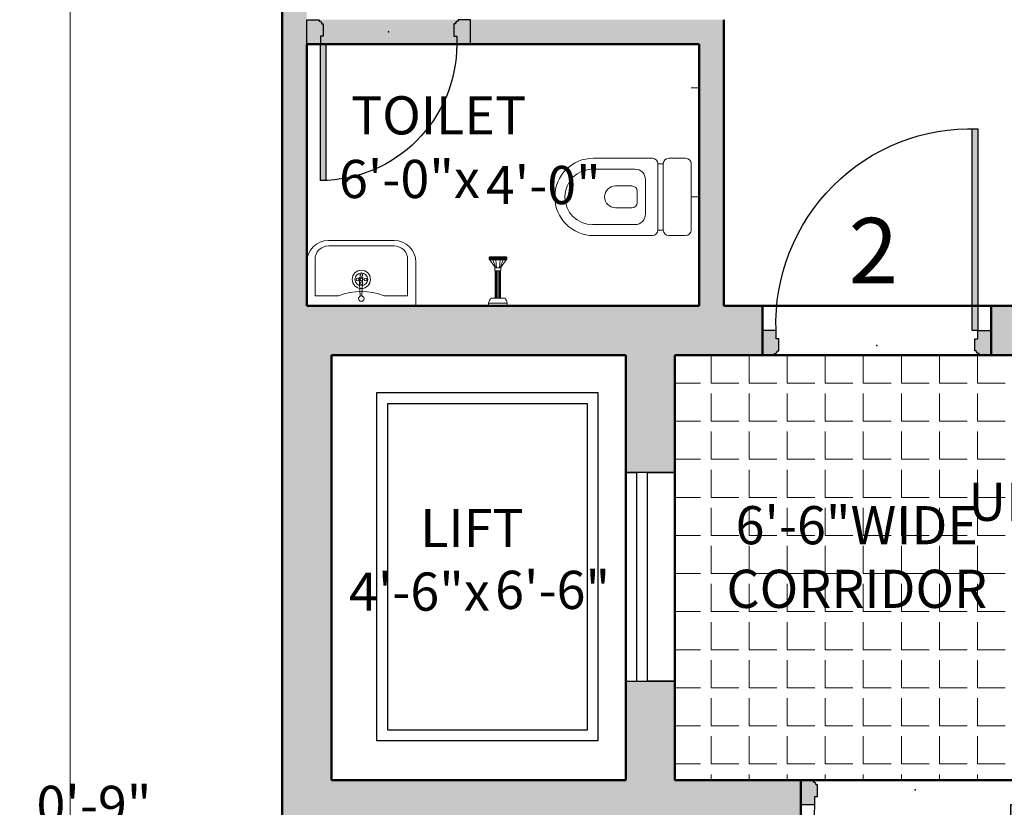
# Model space of a CAD drawing. Units: inches. Extents: x 4508 to 5907, y 877 to 1592.
# Tile 15 of 20: x 5203 to 5383, y 1298 to 1443. Entities that reach past the tile are written whole.
import ezdxf

# ---------------------------------------------------------------- set-up
doc = ezdxf.new("R2010")
doc.units = ezdxf.units.IN
doc.layers.get('DEFPOINTS').update_dxf_attribs({"color": 8})
for name, color, linetype, lineweight in [('A-ANNO-DIMS', 2, 'Continuous', 18), ('A-ANNO-TEXT', 7, 'Continuous', 25), ('A-DOOR', 4, 'Continuous', 25), ('A-EQPM', 6, 'Continuous', 25), ('A-FLOR-FIXT', 8, 'Continuous', 18), ('A-FLOR-PATT', 252, 'Continuous', 13), ('A-WALL', 7, 'Continuous', 50), ('A-WALL-PATT', 8, 'Continuous', 13)]:
    doc.layers.add(name, color=color, linetype=linetype, lineweight=lineweight)
doc.layers.add('doors & windows', color=30, linetype='Continuous')
doc.styles.get("Standard").update_dxf_attribs({"font": 'arial.ttf'})
doc.dimstyles.new('details', dxfattribs={"dimtxt": 5, "dimasz": 2, "dimexe": 2, "dimexo": 3, "dimgap": 1, "dimtad": 0, "dimdec": 1, "dimzin": 0, "dimdsep": 46, "dimlunit": 4, "dimtxsty": 'Standard', "dimblk": 'ARCHTICK', "dimcen": 3, "dimclrd": 256, "dimclre": 256, "dimclrt": 256, "dimadec": 0, "dimazin": 0, "dimtfac": 0.5, "dimtdec": 1, "dimtofl": 0, "dimtmove": 0, "dimatfit": 3, "dimldrblk": 'CLOSEDBLANK', "dimfxl": 2, "dimtolj": 1, "dimtzin": 0, "dimlwd": -1, "dimlwe": -1, "dimarcsym": 0})
doc.dimstyles.new('text', dxfattribs={"dimtxt": 7, "dimasz": 0, "dimexe": 3, "dimexo": 3, "dimgap": 0, "dimtad": 1, "dimtih": 1, "dimtoh": 1, "dimzin": 3, "dimdsep": 46, "dimlunit": 4, "dimtxsty": 'Standard', "dimblk": 'CLOSEDBLANK', "dimcen": 3, "dimse1": 1, "dimse2": 1, "dimsd1": 1, "dimsd2": 1, "dimclrd": 256, "dimclre": 256, "dimclrt": 256, "dimadec": 0, "dimazin": 0, "dimtfac": 0.5, "dimtofl": 0, "dimtmove": 0, "dimatfit": 3, "dimfxl": 3, "dimtolj": 1, "dimtzin": 0, "dimlwd": -1, "dimlwe": -1, "dimarcsym": 0})

# ---------------------------------------------------------------- blocks, each defined once
blk = doc.blocks.new('_ArchTick')
at = {"color": 0, "linetype": 'ByBlock', "const_width": 0.15}
blk.add_lwpolyline([(-0.5, -0.5), (0.5, 0.5)], dxfattribs=at)
blk = doc.blocks.new('*D77')
at = {"layer": 'A-ANNO-DIMS', "color": 0, "transparency": 16777216}
for p, q in [((5201.49, 1574.7), (5213.97, 1574.7)), ((5211.97, 1574.7), (5211.97, 1255.95)), ((5211.97, 926.7), (5211.97, 1245.46)), ((5201.49, 926.7), (5213.97, 926.7))]:
    blk.add_line(p, q, dxfattribs=at)
at = {"layer": 'DEFPOINTS', "color": 0, "transparency": 16777216}
for p in [(5198.49, 1574.7), (5211.97, 1574.7), (5198.49, 926.7)]:
    blk.add_point(p, dxfattribs=at)
at = {"layer": 'A-ANNO-DIMS', "color": 0, "transparency": 16777216, "xscale": 2, "yscale": 2, "zscale": 2}
for p, rotation in [((5211.97, 1574.7), 90), ((5211.97, 926.7), 270)]:
    blk.add_blockref('_ArchTick', p, dxfattribs=dict(at, rotation=rotation))
at = {"layer": 'A-ANNO-DIMS', "color": 0, "transparency": 16777216, "insert": (5211.97, 1250.7), "char_height": 5, "attachment_point": 5, "rotation": 90}
blk.add_mtext("\\A1;54'", dxfattribs=at)
blk = doc.blocks.new('_ClosedBlank')
at = {"color": 0, "lineweight": -2}
for p, q in [((-1, 0.167), (0, 0)), ((-1, 0.167), (-1, -0.167)), ((0, 0), (-1, -0.167))]:
    blk.add_line(p, q, dxfattribs=at)
blk = doc.blocks.new('D2')
at = {"layer": 'doors & windows'}
h = blk.add_hatch(dxfattribs=at)
h.set_pattern_fill('DOTS', color=256, scale=2, angle=180, style=0)
h.set_pattern_definition([(180, (0, -4), (-0.0625, -0.125), [0, -0.125])])
h.paths.add_polyline_path([(2.5, 0), (3.5, 0), (3.5, 24.98, 0.010003), (2.5, 25)])
h = blk.add_hatch(dxfattribs=at)
h.set_pattern_fill('DOTS', color=256, scale=2, angle=180, style=0)
h.set_pattern_definition([(180, (0, 0), (-0.0625, -0.125), [0, -0.125])])
edge = h.paths.add_edge_path()
edge.add_line((27.5, 0), (27.5, -1.5))
edge.add_line((27.5, -1.5), (27, -1.5))
edge.add_line((27, -1.5), (27, -3.75))
edge.add_line((27, -3.75), (27.25, -3.75))
edge.add_arc((27.76, -3.74), 0.509, 181.0059, 268.9941)
edge.add_line((27.75, -4.25), (27.75, -4.5))
edge.add_line((27.75, -4.5), (30, -4.5))
edge.add_line((30, -4.5), (30, 0))
edge.add_line((30, 0), (27.5, 0))
edge = h.paths.add_edge_path()
edge.add_line((2.5, -1.5), (2.5, 0))
edge.add_line((2.5, 0), (0, 0))
edge.add_line((0, 0), (0, -4.5))
edge.add_line((0, -4.5), (2.25, -4.5))
edge.add_line((2.25, -4.5), (2.25, -4.25))
edge.add_arc((2.24, -3.74), 0.509, 271.0059, 358.9941)
edge.add_line((2.75, -3.75), (3, -3.75))
edge.add_line((3, -3.75), (3, -1.5))
edge.add_line((3, -1.5), (2.5, -1.5))
for p, q in [((0, 0), (0, -4.5)), ((30, 0), (30, -4.5))]:
    blk.add_line(p, q)
blk.add_lwpolyline([(3.5, 0), (3.5, 25), (2.5, 25), (2.5, 0)], close=True, dxfattribs=at)
for points in [[(3, -3.75), (3, -1.5), (2.5, -1.5), (2.5, 0), (0, 0)], [(27, -3.75), (27, -1.5), (27.5, -1.5), (27.5, 0), (30, 0)], [(0, -4.5), (2.25, -4.5)], [(30, -4.5), (27.75, -4.5)]]:
    blk.add_lwpolyline(points, dxfattribs=at)
for points in [[(2.25, -4.5), (2.25, -4.25, 0.403966), (2.75, -3.75), (3, -3.75)], [(27.75, -4.5), (27.75, -4.25, -0.403966), (27.25, -3.75), (27, -3.75)]]:
    blk.add_lwpolyline(points, format="xyb", dxfattribs=at)
at = {"layer": 'doors & windows', "ltscale": 6}
blk.add_arc((2.5, 0), 25, 0, 90, dxfattribs=at)
at = {"layer": 'doors & windows'}
blk.add_point((15, -2.25), dxfattribs=at)
blk = doc.blocks.new('commode')
for p, q in [((-7.09, 19.41), (-7.09, 8.61)), ((-5.09, 11.81), (-5.09, 19.57)), ((5.09, 11.81), (5.09, 19.57)), ((7.09, 19.41), (7.09, 8.61)), ((-2, 12.37), (-2, 15.37)), ((2, 12.37), (2, 15.37)), ((-1, 11.37), (1, 11.37)), ((-3.15, 9.87), (3.15, 9.87)), ((-6.09, 7.61), (6.09, 7.61)), ((-6.09, 6.61), (-6.09, 7.61)), ((6.09, 7.61), (6.09, 6.61)), ((-7.09, 2.5), (-7.09, 5.61)), ((-6.09, 6.61), (6.09, 6.61)), ((7.09, 2.5), (7.09, 5.61)), ((-20, 1.5), (-20, 0)), ((-6.09, 1.5), (6.09, 1.5)), ((0, 1.5), (0, 0)), ((20, 1.5), (20, 0))]:
    blk.add_line(p, q)
for centre, radius, start, end in [((0, 19.41), 7.09, 0, 180), ((0, 19.57), 5.09, 0, 180), ((0, 15.37), 2, 0, 180), ((-3.15, 11.81), 1.94, 180, 270), ((-1, 12.37), 1, 180, 270), ((1, 12.37), 1, 270, 0), ((3.15, 11.81), 1.94, 270, 0), ((-6.09, 8.61), 1, 180, 270), ((6.09, 8.61), 1, 270, 0), ((-6.09, 5.61), 1, 90, 180), ((6.09, 5.61), 1, 0, 90), ((-6.09, 2.5), 1, 180, 270), ((6.09, 2.5), 1, 270, 0)]:
    blk.add_arc(centre, radius, start, end)
blk = doc.blocks.new('wash basin 1')
for p, q in [((0, 10), (-8, 10)), ((0, 10), (0, -10)), ((-8.5, 8.5), (-1.85, 8.5)), ((-1.85, 8.5), (-1.85, 4.19)), ((-12, 6), (-12, -6)), ((-11, 6), (-11, -6)), ((-1.85, -8.5), (-1.85, -4.19)), ((-8.5, -8.5), (-1.85, -8.5)), ((0, -10), (-8, -10))]:
    blk.add_line(p, q)
blk.add_lwpolyline([(-1.83, 0.11), (-5.25, 0.25), (-5.23, -0.38), (-1.8, -0.19)])
for centre, radius in [((-4.87, 0), 1.68), ((-4.87, 0), 1.18), ((-5.63, 0), 0.25), ((-4.87, 0.75), 0.25), ((-4.87, 0), 0.25), ((-4.19, 0), 0.25), ((-1.34, 0), 0.5), ((-4.87, -0.72), 0.25)]:
    blk.add_circle(centre, radius)
for centre, radius, start, end in [((-8, 6), 4, 90, 180), ((-8.5, 6), 2.5, 90, 180), ((8.89, 0), 11.53, 158.7059, 201.2941), ((-8, -6), 4, 180, 270), ((-8.5, -6), 2.5, 180, 270)]:
    blk.add_arc(centre, radius, start, end)
blk = doc.blocks.new('tap & shower')
for p, q in [((1.71, 0), (-1.71, 0)), ((-1.71, 0), (-1.71, -0.5)), ((1.71, 0), (1.71, -0.5)), ((1.71, -0.5), (-1.71, -0.5)), ((1.31, -1.4), (-1.31, -1.4)), ((-0.5, -6.44), (-0.5, -1.4)), ((-0.42, -6.44), (-0.42, -1.4)), ((-0.32, -0.5), (0.32, -0.5)), ((-0.3, -6.44), (-0.3, -1.4)), ((-0.14, -6.44), (-0.14, -1.4)), ((0.14, -6.44), (0.14, -1.4)), ((0.3, -6.44), (0.3, -1.4)), ((0.42, -6.44), (0.42, -1.4)), ((0.5, -6.44), (0.5, -1.4)), ((-1.48, -8.46), (-0.47, -6.98)), ((-0.41, -6.98), (-0.94, -8.46)), ((-0.56, -6.44), (0.56, -6.44)), ((-0.56, -6.98), (-0.56, -6.44)), ((-0.56, -6.98), (0.56, -6.98)), ((-0.29, -6.98), (-0.4, -8.46)), ((0.29, -6.98), (0.4, -8.46)), ((0.41, -6.98), (0.94, -8.46)), ((1.48, -8.46), (0.47, -6.98)), ((0.56, -6.98), (0.56, -6.44)), ((-1.62, -8.87), (-1.62, -8.6)), ((-1.48, -8.46), (1.48, -8.46)), ((-1.48, -9), (-1.48, -8.46)), ((-1.48, -9), (1.48, -9)), ((-1.43, -9), (-1.43, -8.46)), ((-1.37, -9), (-1.37, -8.46)), ((-1.32, -9), (-1.32, -8.46)), ((-1.27, -9), (-1.27, -8.46)), ((-1.21, -9), (-1.21, -8.46)), ((-1.16, -9), (-1.16, -8.46)), ((-1.1, -9), (-1.1, -8.46)), ((-1.05, -9), (-1.05, -8.46)), ((-1, -9), (-1, -8.46)), ((-0.94, -9), (-0.94, -8.46)), ((-0.89, -9), (-0.89, -8.46)), ((-0.84, -9), (-0.84, -8.46)), ((-0.78, -9), (-0.78, -8.46)), ((-0.73, -9), (-0.73, -8.46)), ((-0.67, -9), (-0.67, -8.46)), ((-0.62, -9), (-0.62, -8.46)), ((-0.57, -9), (-0.57, -8.46)), ((-0.51, -9), (-0.51, -8.46)), ((-0.46, -9), (-0.46, -8.46)), ((-0.4, -9), (-0.4, -8.46)), ((-0.35, -9), (-0.35, -8.46)), ((-0.3, -9), (-0.3, -8.46)), ((-0.24, -9), (-0.24, -8.46)), ((-0.19, -9), (-0.19, -8.46)), ((-0.13, -9), (-0.13, -8.46)), ((-0.08, -9), (-0.08, -8.46)), ((-0.03, -9), (-0.03, -8.46)), ((0.03, -9), (0.03, -8.46)), ((0.08, -9), (0.08, -8.46)), ((0.13, -9), (0.13, -8.46)), ((0.19, -9), (0.19, -8.46)), ((0.24, -9), (0.24, -8.46)), ((0.3, -9), (0.3, -8.46)), ((0.35, -9), (0.35, -8.46)), ((0.4, -9), (0.4, -8.46)), ((0.46, -9), (0.46, -8.46)), ((0.51, -9), (0.51, -8.46)), ((0.57, -9), (0.57, -8.46)), ((0.62, -9), (0.62, -8.46)), ((0.67, -9), (0.67, -8.46)), ((0.73, -9), (0.73, -8.46)), ((0.78, -9), (0.78, -8.46)), ((0.84, -9), (0.84, -8.46)), ((0.89, -9), (0.89, -8.46)), ((0.94, -9), (0.94, -8.46)), ((1, -9), (1, -8.46)), ((1.05, -9), (1.05, -8.46)), ((1.1, -9), (1.1, -8.46)), ((1.16, -9), (1.16, -8.46)), ((1.21, -9), (1.21, -8.46)), ((1.27, -9), (1.27, -8.46)), ((1.32, -9), (1.32, -8.46)), ((1.37, -9), (1.37, -8.46)), ((1.43, -9), (1.43, -8.46)), ((1.48, -9), (1.48, -8.46)), ((1.62, -8.87), (1.62, -8.6))]:
    blk.add_line(p, q)
for centre, radius, start, end in [((-0.02, -0.29), 1.7, 187.1825, 220.9028), ((0.02, -0.29), 1.7, 319.0972, 352.8175), ((-1.48, -8.6), 0.135, 90, 180), ((-1.48, -8.87), 0.135, 180, 270), ((1.48, -8.6), 0.135, 0, 90), ((1.48, -8.87), 0.135, 270, 0)]:
    blk.add_arc(centre, radius, start, end)
blk = doc.blocks.new('*D86')
at = {"layer": 'DEFPOINTS', "color": 0, "transparency": 16777216}
for p in [(5255.4, 1409.26), (5327.4, 1409.86), (5327.4, 1400.36)]:
    blk.add_point(p, dxfattribs=at)
at = {"layer": 'A-ANNO-DIMS', "color": 0, "transparency": 16777216, "insert": (5274.23, 1419.33), "char_height": 7, "width": 116.2892, "attachment_point": 5}
blk.add_mtext('\\A1;     TOILET\\P6\'-0"x', dxfattribs=at)
blk = doc.blocks.new('*D87')
at = {"layer": 'DEFPOINTS', "color": 0, "transparency": 16777216}
for p in [(5294.13, 1438.2), (5298.79, 1438.2), (5301.15, 1390.2)]:
    blk.add_point(p, dxfattribs=at)
at = {"layer": 'A-ANNO-DIMS', "color": 0, "transparency": 16777216, "insert": (5298.79, 1412.38), "char_height": 7, "attachment_point": 5}
blk.add_mtext('\\A1;4\'-0"', dxfattribs=at)
blk = doc.blocks.new('MD')
at = {"layer": 'doors & windows'}
h = blk.add_hatch(dxfattribs=at)
h.set_pattern_fill('DOTS', color=256, scale=2, style=0)
h.set_pattern_definition([(180, (0, -4), (-0.0625, 0.125), [0, -0.125])])
h.paths.add_polyline_path([(2.5, 37), (3.5, 37), (3.5, 0), (2.5, 0)])
h = blk.add_hatch(dxfattribs=at)
h.set_pattern_fill('DOTS', color=256, scale=2, style=0)
h.set_pattern_definition([(0, (0, -0.5), (0.0625, 0.125), [0, -0.125])])
h.paths.add_polyline_path([(42, -4.5), (42, 0), (39.5, 0), (39.5, -1.5), (39, -1.5), (39, -3.75), (39.25, -3.75, 0.403966), (39.75, -4.25), (39.75, -4.5)])
h.paths.add_polyline_path([(0, -4.5), (2.25, -4.5), (2.25, -4.25, 0.403966), (2.75, -3.75), (3, -3.75), (3, -1.5), (2.5, -1.5), (2.5, 0), (0, 0)])
for p, q in [((0, 0), (0, -4.5)), ((42, 0), (42, -4.5))]:
    blk.add_line(p, q)
blk.add_line((0, -4.5), (2.25, -4.5), dxfattribs=at)
blk.add_lwpolyline([(3.5, 0), (3.5, 37), (2.5, 37), (2.5, 0)], close=True, dxfattribs=at)
for points in [[(3, -3.75), (3, -1.5), (2.5, -1.5), (2.5, 0), (0, 0)], [(39, -3.75), (39, -1.5), (39.5, -1.5), (39.5, 0), (42, 0)], [(42, -4.5), (39.75, -4.5)]]:
    blk.add_lwpolyline(points, dxfattribs=at)
for points in [[(2.25, -4.5), (2.25, -4.25, 0.403966), (2.75, -3.75), (3, -3.75)], [(39.75, -4.5), (39.75, -4.25, -0.403966), (39.25, -3.75), (39, -3.75)]]:
    blk.add_lwpolyline(points, format="xyb", dxfattribs=at)
at = {"layer": 'doors & windows', "ltscale": 6}
blk.add_arc((3.73, 1.23), 35.79, 358.0281, 91.9719, dxfattribs=at)
at = {"layer": 'doors & windows'}
blk.add_point((21, -2.75), dxfattribs=at)
blk = doc.blocks.new('*D90')
at = {"layer": 'DEFPOINTS', "color": 0, "transparency": 16777216}
for p in [(5259.9, 1345.55), (5313.9, 1343.98), (5313.9, 1334.24)]:
    blk.add_point(p, dxfattribs=at)
at = {"layer": 'A-ANNO-DIMS', "color": 0, "transparency": 16777216, "insert": (5276.05, 1343.65), "char_height": 7, "attachment_point": 5}
blk.add_mtext('\\A1;         LIFT\\P4\'-6"x', dxfattribs=at)
blk = doc.blocks.new('*D91')
at = {"layer": 'DEFPOINTS', "color": 0, "transparency": 16777216}
for p in [(5300.5, 1381.2), (5301.11, 1381.2), (5299.95, 1303.2)]:
    blk.add_point(p, dxfattribs=at)
at = {"layer": 'A-ANNO-DIMS', "color": 0, "transparency": 16777216, "insert": (5300.5, 1338.13), "char_height": 7, "attachment_point": 5}
blk.add_mtext('\\A1;6\'-6"', dxfattribs=at)
blk = doc.blocks.new('*D111')
at = {"layer": 'DEFPOINTS', "color": 0, "transparency": 16777216}
for p in [(5355.53, 1383.79), (5355.53, 1305.79), (5356.3, 1305.79)]:
    blk.add_point(p, dxfattribs=at)
at = {"layer": 'A-ANNO-DIMS', "color": 0, "transparency": 16777216, "insert": (5356.3, 1344.16), "char_height": 7, "attachment_point": 5}
blk.add_mtext('\\A1;6\'-6"WIDE \\PCORRIDOR', dxfattribs=at)
blk = doc.blocks.new('*D172')
at = {"layer": 'DEFPOINTS', "color": 0, "transparency": 16777216}
for p in [(5076.25, 1287.03), (5076.25, 1276.01), (5149.75, 1276.01)]:
    blk.add_point(p, dxfattribs=at)
at = {"layer": 'A-ANNO-DIMS', "transparency": 16777216, "insert": (5214.38, 1290.65), "char_height": 7, "attachment_point": 5}
blk.add_mtext('\\A1;DINING TABLE 6\'-1 1/2" TYP.', dxfattribs=at)
blk = doc.blocks.new('*D188')
at = {"layer": 'DEFPOINTS', "color": 0, "transparency": 16777216}
for p in [(5259.90304, 1303.203772), (5216.35304, 1294.203772), (5255.40304, 1294.203772)]:
    blk.add_point(p, dxfattribs=at)
at = {"layer": 'A-ANNO-DIMS', "transparency": 16777216, "insert": (5216.35304, 1298.703772), "char_height": 7, "attachment_point": 5}
blk.add_mtext('\\A1;0\'-9"', dxfattribs=at)

msp = doc.modelspace()

# ---------------------------------------------------------------- hatches: boundary and pattern name
at = {"layer": 'A-FLOR-PATT'}
h = msp.add_hatch(dxfattribs=at)
h.set_pattern_fill('ANGLE', color=256)
h.set_pattern_definition([(0, (0, 0), (0, 6.985), [5.08, -1.905]), (90, (0, 0), (-6.985, 4e-16), [5.08, -1.905])])
h.paths.add_polyline_path([(5397.903, 1339.204, -1), (5397.903, 1345.204), (5397.903, 1381.204), (5387.403, 1381.204), (5322.903, 1381.204), (5322.903, 1303.204), (5397.903, 1303.204)])
h.paths.add_polyline_path([(5327.748, 1331.048), (5384.489, 1331.048), (5384.489, 1357.216), (5327.748, 1357.216)], flags=24)
h.paths.add_polyline_path([(5375.002, 1348.889), (5392.146, 1348.889), (5392.146, 1359.568), (5375.002, 1359.568)], flags=24)
at = {"layer": 'A-WALL-PATT'}
h = msp.add_hatch(color=256, dxfattribs=at)
h.dxf.hatch_style = 1
h.paths.add_polyline_path([(5529.903, 1303.204), (5388.02, 1303.204), (5388.02, 1294.204), (5391.903, 1294.204), (5391.903, 1205.704), (5396.403, 1205.704), (5396.403, 1294.204), (5489.403, 1294.204), (5489.403, 1256.139), (5493.903, 1256.139), (5493.903, 1294.204), (5529.903, 1294.204)], flags=17)
h.paths.add_polyline_path([(5346.02, 1303.204), (5322.903, 1303.204), (5322.903, 1321.388), (5313.903, 1321.388), (5313.903, 1303.204), (5259.903, 1303.204), (5259.903, 1381.204), (5313.903, 1381.204), (5313.903, 1359.674), (5322.903, 1359.674), (5322.903, 1381.204), (5338.979, 1381.204), (5338.979, 1390.204), (5331.903, 1390.204), (5331.903, 1442.704), (5255.403, 1442.704), (5255.403, 1570.204), (5387.403, 1570.204), (5387.403, 1541.271), (5391.903, 1541.271), (5391.903, 1570.204), (5483.403, 1570.204), (5483.403, 1498.204), (5391.903, 1498.204), (5391.903, 1509.559), (5387.403, 1509.559), (5387.403, 1390.204), (5380.979, 1390.204), (5380.979, 1381.204), (5387.403, 1381.204), (5529.903, 1381.204), (5529.903, 1498.204), (5487.903, 1498.204), (5487.903, 1570.204), (5529.903, 1570.204), (5529.903, 1574.704), (5250.903, 1574.704), (5250.903, 991.204), (5310.903, 991.204), (5310.903, 926.704), (5529.903, 926.704), (5529.903, 1210.204), (5525.403, 1210.204), (5525.403, 1103.704), (5499.903, 1103.704), (5499.903, 1210.204), (5493.903, 1210.204), (5493.903, 1256.139), (5489.403, 1256.139), (5489.403, 1210.204), (5461.584, 1210.204), (5461.584, 1205.704), (5495.403, 1205.704), (5495.403, 1103.704), (5436.903, 1103.704), (5436.903, 1051.204), (5391.954, 1051.204), (5391.954, 1103.03), (5391.954, 1107.53), (5255.403, 1108.204), (5255.403, 1294.204), (5346.02, 1294.204)])
h.paths.add_polyline_path([(5255.403, 1390.204), (5255.403, 1398.204), (5255.403, 1438.204), (5257.903, 1438.204), (5258.903, 1438.204), (5327.403, 1438.204), (5327.403, 1390.204), (5325.903, 1390.204)], flags=16)
h.paths.add_polyline_path([(5288.757, 1390.704), (5288.757, 1390.204), (5292.173, 1390.204), (5292.173, 1390.704)], flags=0)
h.paths.add_polyline_path([(5289.965, 1391.606), (5289.965, 1396.645), (5289.903, 1396.645), (5289.903, 1397.319), (5288.849, 1398.862), (5288.849, 1398.8), (5288.983, 1398.748), (5288.983, 1399.204), (5289.091, 1399.204), (5292.081, 1399.204), (5292.081, 1398.665), (5291.946, 1398.665), (5291.027, 1397.319), (5291.027, 1396.645), (5290.965, 1396.645), (5290.965, 1391.606)], flags=0)
h.paths.add_polyline_path([(5288.849, 1399.069, 2.6374395), (5289.056, 1398.835), (5289.117, 1399.087, 0.9346155)], flags=0)
h.paths.add_polyline_path([(5290.061, 1398.665), (5290.061, 1399.204), (5290.038, 1398.975)], flags=0)
h.paths.add_polyline_path([(5291.946, 1398.934, -1), (5291.946, 1398.665)], flags=0)
h.paths.add_polyline_path([(5289.414, 1398.967), (5289.414, 1399.204), (5289.63, 1399.204), (5289.63, 1398.363), (5290.051, 1397.184), (5290.76, 1397.184), (5290.869, 1398.665), (5290.869, 1399.204), (5290.815, 1398.665), (5290.815, 1399.204), (5291.462, 1399.204), (5291.462, 1398.816), (5290.879, 1397.184), (5290.051, 1397.184)], flags=0)
h.paths.add_polyline_path([(5273.903, 1392.056), (5269.591, 1392.056, 0.0901028), (5265.544, 1392.842), (5265.511, 1392.034, -0.3516542), (5265.903, 1391.546, -1), (5264.903, 1391.546, -0.3042165), (5265.213, 1392.008), (5265.167, 1392.84, 0.0880132), (5261.215, 1392.056), (5256.903, 1392.056), (5256.903, 1398.704, -0.4142136), (5259.403, 1401.204), (5271.403, 1401.204, -0.4142136), (5273.903, 1398.704)], flags=0)
h.paths.add_polyline_path([(5263.726, 1395.073, -1), (5267.08, 1395.073, -1)], flags=0)
h.paths.add_polyline_path([(5264.434, 1395.073, -0.695521), (5265.153, 1395.073, -1.1408699), (5265.403, 1395.585, -0.7522125), (5265.403, 1396.25, 0.3674806)], flags=0)
h.paths.add_polyline_path([(5265.153, 1394.399, -1), (5265.653, 1394.399, -1)], flags=0)
h.paths.add_polyline_path([(5265.905, 1395.077, -1), (5266.405, 1395.077, -1)], flags=0)
h.paths.add_polyline_path([(5307.994, 1403.113, -1), (5307.994, 1417.295), (5318.794, 1417.295, -0.4142136), (5319.794, 1416.295), (5320.794, 1416.295, -0.4142136), (5321.794, 1417.295), (5324.903, 1417.295, -0.4142136), (5325.903, 1416.295), (5325.903, 1404.113, -0.4142136), (5324.903, 1403.113), (5321.794, 1403.113, -0.4142136), (5320.794, 1404.113), (5319.794, 1404.113, -0.4142136), (5318.794, 1403.113)], flags=0)
h.paths.add_polyline_path([(5307.836, 1405.113, -1), (5307.836, 1415.295), (5315.591, 1415.295, -0.4142136), (5317.532, 1413.353), (5317.532, 1407.054, -0.4142136), (5315.591, 1405.113)], flags=0)
h.paths.add_polyline_path([(5312.032, 1408.204, -1), (5312.032, 1412.204), (5315.032, 1412.204, -0.4142136), (5316.032, 1411.204), (5316.032, 1409.204, -0.4142136), (5315.032, 1408.204)], flags=0)
h.paths.add_polyline_path([(5391.903, 1385.704), (5391.903, 1493.704), (5525.403, 1493.704), (5525.403, 1385.704)], flags=16)
h.paths.add_polyline_path([(5422.641, 1390.704), (5422.641, 1465.704, -0.9426302), (5422.641, 1467.704), (5494.547, 1467.704, -1), (5494.665, 1465.704), (5494.665, 1390.704, -0.9426302), (5494.665, 1388.704), (5422.759, 1388.704, -1)], flags=0)
h.paths.add_polyline_path([(5427.52, 1395.749, -0.0238564), (5427.614, 1403.949, 0.0884332), (5427.476, 1405.056, 0.0506693), (5427.273, 1405.463, -0.8716827), (5427.713, 1405.835, 0.0268855), (5431.815, 1405.361, 0.0306964), (5436.289, 1405.361, -0.0263641), (5445.798, 1405.259, 0.075811), (5450.408, 1405.53, 0.0687062), (5454.457, 1405.903, -1.0086747), (5454.781, 1405.482, 0.0692081), (5454.389, 1400.959, -0.0519468), (5454.356, 1394.996, 0.1195012), (5454.627, 1392.895, 0.0143508), (5454.796, 1392.489, -0.6962059), (5454.42, 1392.118, 0.1574808), (5448.747, 1392.794, -0.025536), (5432.749, 1392.774, 0.0920085), (5427.781, 1392.048, -0.9384848), (5427.137, 1392.455, 0.0063894), (5427.314, 1392.79, 0.0472995)], flags=0)
h.paths.add_polyline_path([(5426.125, 1411.372, 0.0617649), (5428.641, 1412.201), (5428.641, 1465.704), (5488.665, 1465.704), (5488.665, 1412.363, 0.2363822), (5467.6, 1412.052, -0.2252042)], flags=0)
h.paths.add_polyline_path([(5391.903, 1490.204), (5391.903, 1491.204), (5422.903, 1491.204), (5422.903, 1490.204)], flags=0)
h.paths.add_polyline_path([(5462.545, 1392.771, 0.1270318), (5462.866, 1394.996, -0.0519468), (5462.832, 1400.959, 0.0692081), (5462.441, 1405.482, -1.0086747), (5462.765, 1405.903, 0.0857004), (5471.424, 1405.259, -0.0263641), (5480.932, 1405.361, 0.0306964), (5485.407, 1405.361, 0.0268855), (5489.509, 1405.835, -0.8716827), (5489.949, 1405.463, 0.0506693), (5489.746, 1405.056, 0.0884332), (5489.608, 1403.949, -0.0238564), (5489.702, 1395.749, 0.0472995), (5489.908, 1392.79, 0.0063894), (5490.085, 1392.455, -0.9384848), (5489.441, 1392.048, 0.0920085), (5484.473, 1392.774, -0.025536), (5468.475, 1392.794, 0.1574808), (5462.802, 1392.118, -0.6962059), (5462.426, 1392.489, 0.0100173), (5462.546, 1392.771)], flags=0)
h.paths.add_polyline_path([(5387.454, 1103.03), (5387.454, 1100.53), (5387.454, 1099.53), (5387.454, 995.03), (5387.454, 991.204), (5391.954, 991.204), (5391.954, 1046.704), (5525.403, 1046.704), (5525.403, 931.182), (5391.954, 930.53), (5391.954, 960.53), (5387.454, 960.53), (5387.454, 930.53), (5315.403, 930.53), (5315.403, 991.204), (5323.403, 991.204), (5387.454, 991.204), (5387.454, 995.03), (5255.403, 995.704), (5255.403, 1103.704)], flags=16)
h.paths.add_polyline_path([(5379.264, 1062.889), (5379.264, 1060.156), (5385.764, 1061.889, -0.4526903), (5385.764, 1059.889), (5379.264, 1059.889), (5379.264, 1055.156), (5385.764, 1056.889, -0.4526903), (5385.764, 1054.889), (5379.264, 1054.889), (5379.264, 1050.156), (5385.764, 1051.889, -0.4526903), (5385.764, 1049.889), (5379.264, 1049.889), (5379.264, 1010.156), (5385.764, 1011.889, -0.4526903), (5385.764, 1009.889), (5379.264, 1009.889), (5379.264, 1005.156), (5385.764, 1006.889, -0.4526903), (5385.764, 1004.889), (5379.264, 1004.889), (5379.264, 1000.156), (5385.764, 1001.889, -0.4526903), (5385.764, 999.889), (5378.264, 999.889), (5370.764, 997.889, -0.6674863), (5370.764, 999.889), (5377.264, 999.889), (5377.264, 1004.623), (5370.764, 1002.889, -0.6674863), (5370.764, 1004.889), (5377.264, 1004.889), (5377.264, 1009.623), (5370.764, 1007.889, -0.6674863), (5370.764, 1009.889), (5377.264, 1009.889), (5377.264, 1049.623), (5370.764, 1047.889, -0.6674863), (5370.764, 1049.889), (5377.264, 1049.889), (5377.264, 1054.623), (5370.764, 1052.889, -0.6674863), (5370.764, 1054.889), (5377.264, 1054.889), (5377.264, 1059.623), (5370.764, 1057.889, -0.6674863), (5370.764, 1059.889), (5377.264, 1059.889), (5377.264, 1062.889)], flags=0)
h.paths.add_polyline_path([(5287.641, 1000.704), (5359.665, 1000.704), (5359.665, 1018.212, 0.3202856), (5332.6, 1022.052, -0.246494), (5287.641, 1023.128)], flags=0)
h.paths.add_polyline_path([(5359.547, 1077.704, -1), (5359.665, 1075.704), (5353.665, 1075.704), (5353.665, 1063.704), (5293.641, 1063.704), (5293.641, 1075.704), (5287.759, 1075.704, -1), (5287.641, 1077.704)], flags=0)
h.paths.add_polyline_path([(5441.403, 1099.204), (5525.403, 1099.204), (5525.403, 1051.204), (5441.403, 1051.204), (5441.403, 1059.204)], flags=16)
h.paths.add_polyline_path([(5441.403, 1096.704), (5466.403, 1096.704), (5466.403, 1095.704), (5441.403, 1095.704)], flags=0)
h.paths.add_polyline_path([(5445.403, 1062.204), (5457.403, 1062.204, -0.4142136), (5459.903, 1059.704), (5459.903, 1053.056), (5455.591, 1053.056, 0.0901028), (5451.544, 1053.842), (5451.511, 1053.034, -0.3516542), (5451.903, 1052.546, -1), (5450.903, 1052.546, -0.3042165), (5451.213, 1053.008), (5451.167, 1053.84, 0.0880132), (5447.215, 1053.056), (5442.903, 1053.056), (5442.903, 1059.704, -0.4142136)], flags=0)
h.paths.add_polyline_path([(5453.08, 1056.073, -1), (5449.726, 1056.073, -1)], flags=0)
h.paths.add_polyline_path([(5292.713, 1015.835, 0.0268855), (5296.815, 1015.361, 0.0306964), (5301.289, 1015.361, -0.0263641), (5310.798, 1015.259, 0.075811), (5315.408, 1015.53, 0.0687062), (5319.457, 1015.903, -1.0086747), (5319.781, 1015.482, 0.0692081), (5319.389, 1010.959, -0.0519468), (5319.356, 1004.996, 0.1195012), (5319.627, 1002.895, 0.0143508), (5319.796, 1002.489, -0.6962059), (5319.42, 1002.118, 0.1574808), (5313.747, 1002.794, -0.025536), (5297.749, 1002.774, 0.0920085), (5292.781, 1002.048, -0.9384848), (5292.137, 1002.455, 0.0063894), (5292.314, 1002.79, 0.0472995), (5292.52, 1005.749, -0.0238564), (5292.614, 1013.949, 0.0884332), (5292.476, 1015.056, 0.0506693), (5292.273, 1015.463, -0.8716827)], flags=0)
h.paths.add_polyline_path([(5450.434, 1056.073, -0.695521), (5451.153, 1056.073, -1.1408699), (5451.403, 1056.585, -0.7522125), (5451.403, 1057.25, 0.3674806)], flags=0)
h.paths.add_polyline_path([(5327.765, 1015.903, 0.0857004), (5336.424, 1015.259, -0.0263641), (5345.932, 1015.361, 0.0306964), (5350.407, 1015.361, 0.0268855), (5354.509, 1015.835, -0.8716827), (5354.949, 1015.463, 0.0506693), (5354.746, 1015.056, 0.0884332), (5354.608, 1013.949, -0.0238564), (5354.702, 1005.749, 0.0472995), (5354.908, 1002.79, 0.0063894), (5355.085, 1002.455, -0.9384848), (5354.441, 1002.048, 0.0920085), (5349.473, 1002.774, -0.025536), (5333.475, 1002.794, 0.1574808), (5327.802, 1002.118, -0.6962059), (5327.426, 1002.489, 0.0100173), (5327.546, 1002.771), (5327.545, 1002.771, 0.1270318), (5327.866, 1004.996, -0.0519468), (5327.832, 1010.959, 0.0692081), (5327.441, 1015.482, -1.0086747)], flags=0)
h.paths.add_polyline_path([(5452.405, 1056.077, -1), (5451.905, 1056.077, -1)], flags=0)
h.paths.add_polyline_path([(5451.653, 1055.399, -1), (5451.153, 1055.399, -1)], flags=0)
h.paths.add_polyline_path([(5472.958, 1051.704), (5472.958, 1051.204), (5476.374, 1051.204), (5476.374, 1051.704)], flags=0)
h.paths.add_polyline_path([(5476.282, 1060.204), (5476.282, 1059.665), (5476.147, 1059.665), (5475.228, 1058.319), (5475.228, 1057.645), (5475.166, 1052.606), (5474.166, 1052.606), (5474.166, 1057.645), (5474.104, 1057.645), (5474.104, 1058.319), (5473.05, 1059.862), (5473.05, 1059.8), (5473.184, 1059.748), (5473.184, 1060.204), (5473.292, 1060.204)], flags=0)
h.paths.add_polyline_path([(5473.05, 1060.069, 2.6374395), (5473.257, 1059.835), (5473.318, 1060.087, 0.9346155)], flags=0)
h.paths.add_polyline_path([(5473.831, 1060.204), (5473.831, 1059.363), (5474.252, 1058.184), (5474.371, 1058.184), (5474.262, 1059.665), (5474.262, 1060.204)], flags=0)
h.paths.add_polyline_path([(5475.501, 1060.204), (5475.501, 1059.363), (5475.555, 1059.514), (5475.555, 1060.204)], flags=0)
h.paths.add_polyline_path([(5474.855, 1060.204), (5474.908, 1060.127), (5474.908, 1060.204), (5474.855, 1059.665)], flags=0)
h.paths.add_polyline_path([(5476.147, 1059.934, -1), (5476.147, 1059.665)], flags=0)
h.paths.add_polyline_path([(5474.693, 1060.204), (5475.178, 1059.511), (5475.178, 1060.204), (5475.285, 1059.934), (5475.285, 1060.204), (5475.178, 1059.665), (5475.178, 1060.204), (5475.07, 1059.665), (5475.07, 1060.204), (5474.962, 1059.665), (5474.962, 1060.204), (5474.693, 1059.306)], flags=0)
h.paths.add_polyline_path([(5474.747, 1060.204), (5474.37, 1059.45), (5474.37, 1060.204), (5474.424, 1060.096), (5474.424, 1060.204), (5474.747, 1059.665)], flags=0)
h.paths.add_polyline_path([(5476.04, 1059.665), (5476.04, 1060.204), (5476.094, 1059.665), (5476.094, 1060.204)], flags=0)
h.paths.add_polyline_path([(5505.994, 1082.295), (5516.794, 1082.295, -0.4142136), (5517.794, 1081.295), (5518.794, 1081.295, -0.4142136), (5519.794, 1082.295), (5522.903, 1082.295, -0.4142136), (5523.903, 1081.295), (5523.903, 1069.113, -0.4142136), (5522.903, 1068.113), (5519.794, 1068.113, -0.4142136), (5518.794, 1069.113), (5517.794, 1069.113, -0.4142136), (5516.794, 1068.113), (5505.994, 1068.113, -1)], flags=0)
h.paths.add_polyline_path([(5505.836, 1080.295), (5513.591, 1080.295, -0.4142136), (5515.532, 1078.353), (5515.532, 1072.054, -0.4142136), (5513.591, 1070.113), (5505.836, 1070.113, -1)], flags=0)
h.paths.add_polyline_path([(5520.403, 963.695), (5520.403, 1035.72), (5502.895, 1035.72, 0.3202856), (5499.055, 1008.654, -0.246494), (5497.978, 963.695)], flags=0)
h.paths.add_polyline_path([(5445.403, 1035.72), (5445.403, 1029.72), (5457.403, 1029.72), (5457.403, 969.695), (5445.403, 969.695), (5445.403, 963.814, -1), (5443.403, 963.695), (5443.403, 1035.602, -1)], flags=0)
h.paths.add_polyline_path([(5510.032, 1077.204), (5513.032, 1077.204, -0.4142136), (5514.032, 1076.204), (5514.032, 1074.204, -0.4142136), (5513.032, 1073.204), (5510.032, 1073.204, -1)], flags=0)
h.paths.add_polyline_path([(5317.255, 989.704), (5323.903, 989.704, -0.4142136), (5326.403, 987.204), (5326.403, 975.204, -0.4142136), (5323.903, 972.704), (5317.255, 972.704), (5317.255, 977.016, 0.0901028), (5318.041, 981.063), (5317.233, 981.096, -0.8964437), (5316.245, 981.204, -0.8220123), (5317.207, 981.394), (5318.04, 981.44, 0.0880132), (5317.255, 985.392)], flags=0)
h.paths.add_polyline_path([(5321.949, 981.204, -1), (5318.594, 981.204, -1)], flags=0)
h.paths.add_polyline_path([(5362.454, 988.03), (5387.454, 988.03), (5387.454, 990.53), (5391.954, 990.53), (5391.704, 988.289, -0.4090807), (5391.204, 987.78), (5391.204, 987.53), (5388.954, 987.53), (5388.954, 988.03), (5387.454, 988.03), (5387.454, 987.03), (5362.474, 987.03, 0.4025427), (5387.454, 963.03), (5388.954, 963.03), (5388.954, 963.53), (5391.195, 963.28, -0.4142136), (5391.704, 962.771), (5391.954, 960.53), (5391.954, 962.78), (5391.704, 962.78, 0.4090807), (5391.195, 963.28), (5388.954, 963.53), (5388.954, 963.03), (5387.454, 963.03, -0.4025427), (5362.474, 987.03), (5362.454, 987.03)], flags=0)
h.paths.add_polyline_path([(5321.285, 981.204, -0.6555366), (5320.522, 981.204, -1.1195284), (5320.275, 980.701, -1.3500746), (5320.279, 980.026, 0.3749463)], flags=0)
h.paths.add_polyline_path([(5320.022, 981.923, -1), (5320.522, 981.923, -1)], flags=0)
h.paths.add_polyline_path([(5319.348, 981.204, -1), (5319.848, 981.204, -1)], flags=0)
h.paths.add_polyline_path([(5507.157, 1030.662, -0.0238564), (5515.358, 1030.756, 0.0472995), (5518.317, 1030.962, 0.0063894), (5518.652, 1031.139, -0.9384848), (5519.059, 1030.495, 0.0920085), (5518.333, 1025.527, -0.025536), (5518.313, 1009.53, 0.1574808), (5518.989, 1003.857, -0.6962059), (5518.618, 1003.48, 0.0100173), (5518.335, 1003.601), (5518.335, 1003.6, 0.1270318), (5516.111, 1003.921, -0.0519468), (5510.148, 1003.887, 0.0692081), (5505.624, 1003.495, -1.0086747), (5505.204, 1003.819, 0.0857004), (5505.848, 1012.479, -0.0263641), (5505.746, 1021.987, 0.0306964), (5505.746, 1026.462, 0.0268855), (5505.272, 1030.563, -0.8716827), (5505.644, 1031.004, 0.0506693), (5506.051, 1030.801, 0.0884332)], flags=0)
h.paths.add_polyline_path([(5368.045, 945.621), (5378.845, 945.621, -0.4142136), (5379.845, 944.621), (5380.845, 944.621, -0.4142136), (5381.845, 945.621), (5384.954, 945.621, -0.4142136), (5385.954, 944.621), (5385.954, 932.439, -0.4142136), (5384.954, 931.439), (5381.845, 931.439, -0.4142136), (5380.845, 932.439), (5379.845, 932.439, -0.4142136), (5378.845, 931.439), (5368.045, 931.439, -1)], flags=0)
h.paths.add_polyline_path([(5327.31, 931.03), (5327.31, 930.53), (5330.726, 930.53), (5330.726, 931.03)], flags=0)
h.paths.add_polyline_path([(5330.634, 939.53), (5330.634, 938.991), (5330.499, 938.991), (5329.579, 937.645), (5329.579, 936.971), (5329.518, 936.971), (5329.518, 931.933), (5328.518, 931.933), (5328.518, 936.971), (5328.456, 936.971), (5328.456, 937.645), (5327.402, 939.189), (5327.402, 939.126), (5327.536, 939.074), (5327.536, 939.53), (5327.644, 939.53)], flags=0)
h.paths.add_polyline_path([(5327.402, 939.395, 2.6374395), (5327.609, 939.161), (5327.67, 939.414, 0.9346155)], flags=0)
h.paths.add_polyline_path([(5328.021, 939.142), (5328.021, 939.53), (5327.967, 939.53), (5327.967, 939.293)], flags=0)
h.paths.add_polyline_path([(5328.614, 939.53), (5328.614, 938.991), (5328.723, 937.51), (5329.313, 937.51), (5329.422, 938.991), (5329.422, 939.53), (5329.368, 938.991), (5329.368, 939.53)], flags=0)
h.paths.add_polyline_path([(5329.853, 939.53), (5329.853, 938.689), (5329.907, 938.84), (5329.907, 939.53)], flags=0)
h.paths.add_polyline_path([(5330.499, 939.261, -1), (5330.499, 938.991)], flags=0)
h.paths.add_polyline_path([(5367.887, 943.621), (5375.641, 943.621, -0.4142136), (5377.583, 941.68), (5377.583, 935.38, -0.4142136), (5375.641, 933.439), (5367.887, 933.439, -1)], flags=0)
h.paths.add_polyline_path([(5509.267, 947.14), (5509.267, 939.64), (5511.267, 932.14, -0.4526903), (5509.267, 932.14), (5509.267, 938.64), (5504.534, 938.64), (5506.267, 932.14, -0.4526903), (5504.267, 932.14), (5504.267, 938.64), (5499.534, 938.64), (5501.267, 932.14, -0.4526903), (5499.267, 932.14), (5499.267, 938.64), (5459.534, 938.64), (5461.267, 932.14, -0.4526903), (5459.267, 932.14), (5459.267, 938.64), (5454.534, 938.64), (5456.267, 932.14, -0.4526903), (5454.267, 932.14), (5454.267, 938.64), (5449.534, 938.64), (5451.267, 932.14, -0.4526903), (5449.267, 932.14), (5449.267, 939.64), (5447.267, 947.14, -0.3030853), (5448.267, 947.808), (5508.266, 947.808, -0.3032033)], flags=0)
h.paths.add_polyline_path([(5510.148, 995.444, -0.0519468), (5516.111, 995.41, 0.1195012), (5518.212, 995.681, 0.0143508), (5518.618, 995.851, -0.6962059), (5518.989, 995.474, 0.1574808), (5518.313, 989.801, -0.025536), (5518.333, 973.804, 0.0920085), (5519.059, 968.836, -0.9384848), (5518.652, 968.192, 0.0063894), (5518.317, 968.369, 0.0472995), (5515.358, 968.575, -0.0238564), (5507.157, 968.669, 0.0884332), (5506.051, 968.531, 0.0506693), (5505.644, 968.327, -0.8716827), (5505.272, 968.768, 0.0268855), (5505.746, 972.869, 0.0306964), (5505.746, 977.344, -0.0263641), (5505.848, 986.852, 0.075811), (5505.576, 991.462, 0.0687062), (5505.204, 995.512, -1.0086747), (5505.624, 995.836, 0.0692081)], flags=0)
h.paths.add_polyline_path([(5372.083, 940.53), (5375.083, 940.53, -0.4142136), (5376.083, 939.53), (5376.083, 937.53, -0.4142136), (5375.083, 936.53), (5372.083, 936.53, -1)], flags=0)
h.paths.add_polyline_path([(5409.258, 1465.643), (5487.738, 1465.643), (5487.738, 1492.394), (5409.258, 1492.394)], flags=8)
h.paths.add_polyline_path([(5463.574, 1465.103), (5486.546, 1465.103), (5486.546, 1479.528), (5463.574, 1479.528)], flags=8)
h.paths.add_polyline_path([(5248.665, 1406.171), (5299.981, 1406.171), (5299.981, 1432.34), (5248.665, 1432.34)], flags=9)
h.paths.add_polyline_path([(5287.471, 1405.121), (5310.443, 1405.121), (5310.443, 1419.546), (5287.471, 1419.546)], flags=8)
h.paths.add_polyline_path([(5371.637, 1047.927), (5371.637, 1010.764), (5377.841, 1010.764), (5377.841, 1047.927)], flags=8)
h.paths.add_polyline_path([(5324.882, 1074.869), (5347.854, 1074.869), (5347.854, 1089.294), (5324.882, 1089.294)], flags=8)
h.paths.add_polyline_path([(5262.863, 1074.665), (5351.123, 1074.665), (5351.123, 1100.833), (5262.863, 1100.833)], flags=8)
h.paths.add_polyline_path([(5307.238, 938.814), (5363.988, 938.814), (5363.988, 964.982), (5307.238, 964.982)], flags=24)
h.paths.add_polyline_path([(5348.837, 937.997), (5371.809, 937.997), (5371.809, 952.422), (5348.837, 952.422)], flags=8)
h.paths.add_polyline_path([(5432.497, 1066.695), (5489.247, 1066.695), (5489.247, 1092.863), (5432.497, 1092.863)], flags=24)
h.paths.add_polyline_path([(5473.52, 1065.943), (5496.492, 1065.943), (5496.492, 1080.368), (5473.52, 1080.368)], flags=8)
h.paths.add_polyline_path([(5451.783, 984.266), (5480.194, 984.266), (5480.194, 998.691), (5451.783, 998.691)], flags=8)
h.paths.add_polyline_path([(5392.211, 983.632), (5481.554, 983.632), (5481.554, 1010.383), (5392.211, 1010.383)], flags=8)
h.paths.add_polyline_path([(5497.304, 946.267), (5460.142, 946.267), (5460.142, 940.062), (5497.304, 940.062)], flags=8)

# ---------------------------------------------------------------- linework, layer by layer
at = {"layer": 'A-EQPM'}
for points in [[(5308.818, 1310.432), (5268.276, 1310.432), (5268.276, 1374.324), (5308.818, 1374.324)], [(5306.818, 1312.432), (5270.276, 1312.432), (5270.276, 1372.324), (5306.818, 1372.324)]]:
    msp.add_lwpolyline(points, close=True, dxfattribs=at)
msp.add_lwpolyline([(5313.903, 1321.388), (5322.903, 1321.388), (5317.903, 1321.388), (5317.903, 1359.674), (5322.903, 1359.674), (5313.903, 1359.674), (5315.903, 1359.674), (5315.903, 1321.388)], dxfattribs=at)
at = {"layer": 'A-WALL'}
for p, q in [((5250.903, 926.704), (5250.903, 1574.704)), ((5331.903, 1390.204), (5331.903, 1442.704)), ((5255.403, 1438.204), (5327.403, 1438.204)), ((5255.403, 1390.204), (5255.403, 1438.204)), ((5327.403, 1390.204), (5327.403, 1438.204)), ((5255.403, 1390.204), (5327.403, 1390.204)), ((5331.903, 1390.204), (5387.403, 1390.204)), ((5259.903, 1381.204), (5313.903, 1381.204)), ((5259.903, 1303.204), (5259.903, 1381.204)), ((5313.903, 1303.204), (5313.903, 1381.204)), ((5322.903, 1303.204), (5322.903, 1381.204)), ((5322.903, 1381.204), (5387.403, 1381.204)), ((5259.903, 1303.204), (5313.903, 1303.204)), ((5322.903, 1303.204), (5529.903, 1303.204)), ((5346.02, 1303.204), (5346.02, 1294.204))]:
    msp.add_line(p, q, dxfattribs=at)
for points in [[(5338.979, 1381.204), (5338.979, 1390.204)], [(5380.979, 1381.204), (5380.979, 1390.204)]]:
    msp.add_lwpolyline(points, dxfattribs=at)

# ---------------------------------------------------------------- block references
at = {"layer": 'A-DOOR', "xscale": -1, "rotation": 180}
msp.add_blockref('D2', (5255.403, 1438.204), dxfattribs=at)
at = {"layer": 'A-DOOR', "xscale": -1}
msp.add_blockref('MD', (5380.979, 1385.704), dxfattribs=at)
at = {"layer": 'A-DOOR', "rotation": 180}
msp.add_blockref('MD', (5388.02, 1298.704), dxfattribs=at)
at = {"layer": 'A-FLOR-FIXT'}
for name, p, rotation in [('commode', (5327.403, 1410.204), 90), ('wash basin 1', (5265.403, 1390.204), 270)]:
    msp.add_blockref(name, p, dxfattribs=dict(at, rotation=rotation))
at = {"layer": 'A-FLOR-FIXT', "xscale": -1, "rotation": 180}
msp.add_blockref('tap & shower', (5290.465, 1390.204), dxfattribs=at)

# ---------------------------------------------------------------- texts
at = {"layer": 'A-ANNO-TEXT'}
for s, height, p in [('2', 12, (5354.802, 1394.353)), ('UP', 7, (5376.782, 1350.788))]:
    msp.add_text(s, height=height, dxfattribs=at).set_placement(p)

# ---------------------------------------------------------------- dimensions: what is measured, and where the dimension line sits
at = {"layer": 'A-ANNO-DIMS'}
for base, p1, p2, dimstyle, override, picture, middle in [((5211.971, 1574.704), (5198.492, 926.704), (5198.492, 1574.704), 'details', {"dimclrd": 0, "dimclre": 0, "dimclrt": 0}, '*D77', (5211.971, 1250.704)), ((5216.353, 1294.204), (5259.903, 1303.204), (5255.403, 1294.204), 'text', {"dimdec": 1, "dimlfac": 1, "dimrnd": 0, "dimzin": 1, "dimdsep": 46, "dimlunit": 4, "dimfrac": 2}, '*D188', (5216.353, 1298.704))]:
    dim = msp.add_linear_dim(base=base, p1=p1, p2=p2, angle=90, dimstyle=dimstyle, override=override, dxfattribs=at)
    dim.commit()
    dim.dimension.update_dxf_attribs({"geometry": picture, "text_midpoint": middle})
for base, p1, p2, angle, override, picture, middle in [((5298.79, 1438.204), (5301.146, 1390.204), (5294.126, 1438.204), 90, {"dimtad": 0, "dimclrd": 0, "dimclre": 0, "dimclrt": 0}, '*D87', (5298.79, 1412.384)), ((5300.498, 1381.204), (5299.952, 1303.204), (5301.107, 1381.204), 270, {"dimclrd": 0, "dimclre": 0, "dimclrt": 0}, '*D91', (5300.498, 1338.134))]:
    dim = msp.add_linear_dim(base=base, p1=p1, p2=p2, angle=angle, dimstyle='text', override=override, dxfattribs=at)
    dim.commit()
    dim.dimension.update_dxf_attribs({"geometry": picture, "text_midpoint": middle, "dimtype": 160})
for base, p1, p2, text, picture, middle in [((5327.403, 1409.86), (5255.403, 1409.262), (5327.403, 1400.356), '     TOILET\\P<>x', '*D86', (5274.225, 1409.86)), ((5313.903, 1334.241), (5259.903, 1345.554), (5313.903, 1343.978), '         LIFT\\P<>x', '*D90', (5276.047, 1334.241))]:
    dim = msp.add_linear_dim(base=base, p1=p1, p2=p2, text=text, dimstyle='text', override={"dimclrd": 0, "dimclre": 0, "dimclrt": 0}, dxfattribs=at)
    dim.commit()
    dim.dimension.update_dxf_attribs({"geometry": picture, "text_midpoint": middle, "dimtype": 160})
dim = msp.add_linear_dim(base=(5356.3, 1305.792), p1=(5355.527, 1383.792), p2=(5355.527, 1305.792), angle=90, text='<>WIDE \\PCORRIDOR', dimstyle='text', override={"dimtad": 0, "dimclrd": 0, "dimclre": 0, "dimclrt": 0}, dxfattribs=at)
dim.commit()
dim.dimension.update_dxf_attribs({"geometry": '*D111', "text_midpoint": (5356.3, 1344.158), "dimtype": 160})
dim = msp.add_linear_dim(base=(5076.246, 1287.034), p1=(5149.746, 1276.009), p2=(5076.246, 1276.009), angle=180, text='DINING TABLE <> TYP.', dimstyle='text', override={"dimdec": 1, "dimrnd": 0, "dimzin": 1, "dimlunit": 4, "dimfrac": 2}, dxfattribs=at)
dim.commit()
dim.dimension.update_dxf_attribs({"geometry": '*D172', "text_midpoint": (5214.381, 1290.653)})

doc.saveas('drawing.dxf')
